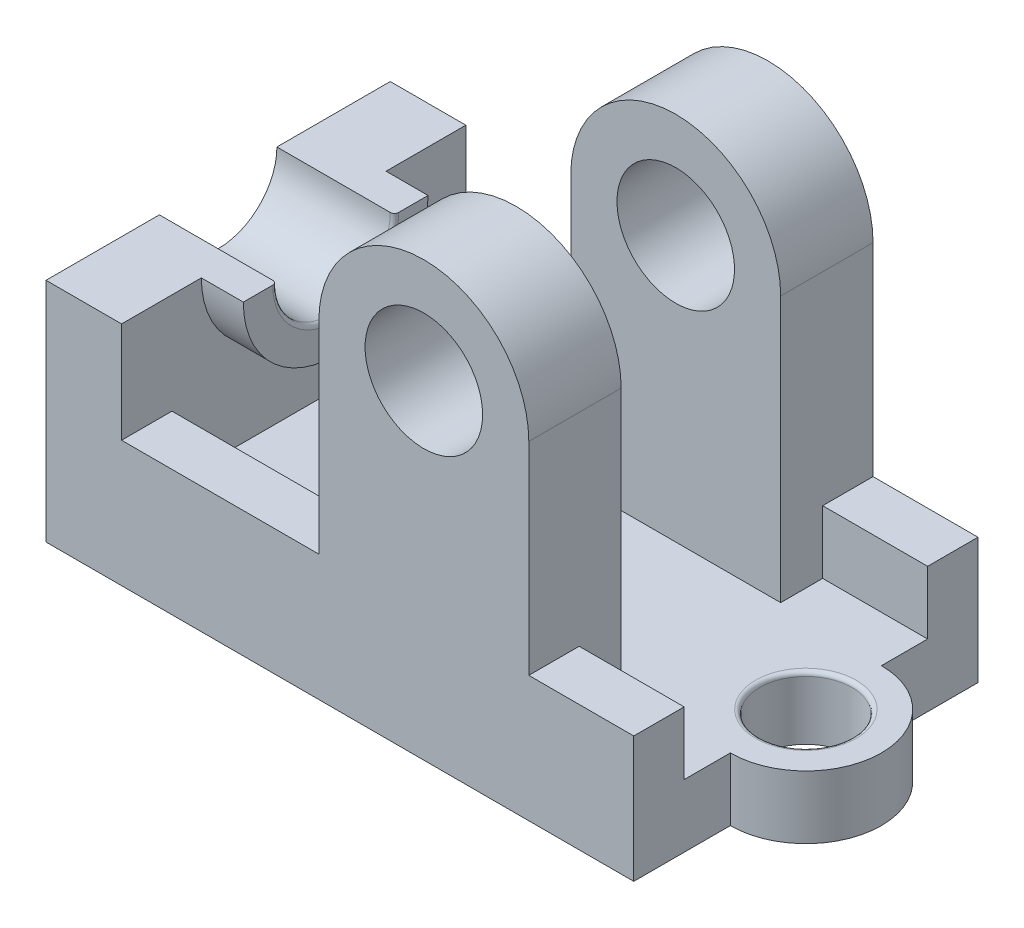
ISO-10303-21;
HEADER;
FILE_DESCRIPTION(('STEP AP214'),'2;1');
FILE_NAME('part.step','',(''),(''),'','','');
FILE_SCHEMA(('AUTOMOTIVE_DESIGN { 1 0 10303 214 1 1 1 1 }'));
ENDSEC;
DATA;
#1=APPLICATION_CONTEXT('core data for automotive mechanical design processes');
#2=APPLICATION_PROTOCOL_DEFINITION('international standard','automotive_design',2000,#1);
#3=PRODUCT_CONTEXT('',#1,'mechanical');
#4=PRODUCT('Part','Part','',(#3));
#5=PRODUCT_RELATED_PRODUCT_CATEGORY('part','',(#4));
#6=PRODUCT_DEFINITION_FORMATION('','',#4);
#7=PRODUCT_DEFINITION_CONTEXT('part definition',#1,'design');
#8=PRODUCT_DEFINITION('design','',#6,#7);
#9=PRODUCT_DEFINITION_SHAPE('','',#8);
#10=(LENGTH_UNIT() NAMED_UNIT(*) SI_UNIT(.MILLI.,.METRE.));
#11=(NAMED_UNIT(*) PLANE_ANGLE_UNIT() SI_UNIT($,.RADIAN.));
#12=(NAMED_UNIT(*) SI_UNIT($,.STERADIAN.) SOLID_ANGLE_UNIT());
#13=UNCERTAINTY_MEASURE_WITH_UNIT(LENGTH_MEASURE(1.E-05),#10,'distance_accuracy_value','');
#14=(GEOMETRIC_REPRESENTATION_CONTEXT(3) GLOBAL_UNCERTAINTY_ASSIGNED_CONTEXT((#13)) GLOBAL_UNIT_ASSIGNED_CONTEXT((#10,
#11,#12)) REPRESENTATION_CONTEXT('',''));
#15=CARTESIAN_POINT('',(0.,0.,0.));
#16=DIRECTION('',(0.,0.,1.));
#17=DIRECTION('',(1.,0.,0.));
#18=AXIS2_PLACEMENT_3D('',#15,#16,#17);
#19=CARTESIAN_POINT('',(0.,54.,0.));
#20=DIRECTION('',(0.,1.,0.));
#21=DIRECTION('',(0.,0.,1.));
#22=AXIS2_PLACEMENT_3D('',#19,#20,#21);
#23=PLANE('',#22);
#24=DIRECTION('',(-1.,0.,0.));
#25=VECTOR('',#24,1.);
#26=CARTESIAN_POINT('',(-48.,54.,-14.));
#27=LINE('',#26,#25);
#28=CARTESIAN_POINT('',(-43.,54.,-14.));
#29=VERTEX_POINT('',#28);
#30=CARTESIAN_POINT('',(-70.,54.,-14.));
#31=VERTEX_POINT('',#30);
#32=EDGE_CURVE('E460',#29,#31,#27,.T.);
#33=ORIENTED_EDGE('',*,*,#32,.F.);
#34=CARTESIAN_POINT('',(-43.,54.,-15.));
#35=DIRECTION('',(0.,1.,0.));
#36=DIRECTION('',(0.,0.,1.));
#37=AXIS2_PLACEMENT_3D('',#34,#35,#36);
#38=CIRCLE('',#37,1.);
#39=CARTESIAN_POINT('',(-42.,54.,-15.));
#40=VERTEX_POINT('',#39);
#41=EDGE_CURVE('E68',#29,#40,#38,.T.);
#42=ORIENTED_EDGE('',*,*,#41,.T.);
#43=DIRECTION('',(0.,0.,-1.));
#44=VECTOR('',#43,1.);
#45=CARTESIAN_POINT('',(-42.,54.,-14.));
#46=LINE('',#45,#44);
#47=CARTESIAN_POINT('',(-42.,54.,-22.));
#48=VERTEX_POINT('',#47);
#49=EDGE_CURVE('E234',#40,#48,#46,.T.);
#50=ORIENTED_EDGE('',*,*,#49,.T.);
#51=DIRECTION('',(-1.,0.,0.));
#52=VECTOR('',#51,1.);
#53=CARTESIAN_POINT('',(-42.,54.,-22.));
#54=LINE('',#53,#52);
#55=CARTESIAN_POINT('',(-52.,54.,-22.));
#56=VERTEX_POINT('',#55);
#57=EDGE_CURVE('E236',#48,#56,#54,.T.);
#58=ORIENTED_EDGE('',*,*,#57,.T.);
#59=DIRECTION('',(0.,0.,-1.));
#60=VECTOR('',#59,1.);
#61=CARTESIAN_POINT('',(-52.,54.,-41.));
#62=LINE('',#61,#60);
#63=CARTESIAN_POINT('',(-52.,54.,-41.));
#64=VERTEX_POINT('',#63);
#65=EDGE_CURVE('E388',#56,#64,#62,.T.);
#66=ORIENTED_EDGE('',*,*,#65,.T.);
#67=DIRECTION('',(-1.,0.,0.));
#68=VECTOR('',#67,1.);
#69=CARTESIAN_POINT('',(-70.,54.,-41.));
#70=LINE('',#69,#68);
#71=CARTESIAN_POINT('',(-70.,54.,-41.));
#72=VERTEX_POINT('',#71);
#73=EDGE_CURVE('E392',#64,#72,#70,.T.);
#74=ORIENTED_EDGE('',*,*,#73,.T.);
#75=DIRECTION('',(0.,0.,1.));
#76=VECTOR('',#75,1.);
#77=CARTESIAN_POINT('',(-70.,54.,-41.));
#78=LINE('',#77,#76);
#79=EDGE_CURVE('E381',#72,#31,#78,.T.);
#80=ORIENTED_EDGE('',*,*,#79,.T.);
#81=EDGE_LOOP('',(#33,#42,#50,#58,#66,#74,#80));
#82=FACE_BOUND('',#81,.T.);
#83=ADVANCED_FACE('F44',(#82),#23,.T.);
#84=CARTESIAN_POINT('',(-52.,30.,-29.));
#85=DIRECTION('',(0.,0.,-1.));
#86=DIRECTION('',(-1.,0.,0.));
#87=AXIS2_PLACEMENT_3D('',#84,#85,#86);
#88=PLANE('',#87);
#89=DIRECTION('',(1.,0.,0.));
#90=VECTOR('',#89,1.);
#91=CARTESIAN_POINT('',(-52.,15.,-29.));
#92=LINE('',#91,#90);
#93=CARTESIAN_POINT('',(-52.,15.,-29.));
#94=VERTEX_POINT('',#93);
#95=CARTESIAN_POINT('',(-5.,15.,-29.));
#96=VERTEX_POINT('',#95);
#97=EDGE_CURVE('E362',#94,#96,#92,.T.);
#98=ORIENTED_EDGE('',*,*,#97,.T.);
#99=DIRECTION('',(0.,1.,0.));
#100=VECTOR('',#99,1.);
#101=CARTESIAN_POINT('',(-5.,30.,-29.));
#102=LINE('',#101,#100);
#103=CARTESIAN_POINT('',(-5.,30.,-29.));
#104=VERTEX_POINT('',#103);
#105=EDGE_CURVE('E290',#96,#104,#102,.T.);
#106=ORIENTED_EDGE('',*,*,#105,.T.);
#107=DIRECTION('',(1.,0.,0.));
#108=VECTOR('',#107,1.);
#109=CARTESIAN_POINT('',(-52.,30.,-29.));
#110=LINE('',#109,#108);
#111=CARTESIAN_POINT('',(-52.,30.,-29.));
#112=VERTEX_POINT('',#111);
#113=EDGE_CURVE('E366',#112,#104,#110,.T.);
#114=ORIENTED_EDGE('',*,*,#113,.F.);
#115=DIRECTION('',(0.,-1.,0.));
#116=VECTOR('',#115,1.);
#117=CARTESIAN_POINT('',(-52.,30.,-29.));
#118=LINE('',#117,#116);
#119=EDGE_CURVE('E379',#112,#94,#118,.T.);
#120=ORIENTED_EDGE('',*,*,#119,.T.);
#121=EDGE_LOOP('',(#98,#106,#114,#120));
#122=FACE_BOUND('',#121,.T.);
#123=ADVANCED_FACE('F481',(#122),#88,.F.);
#124=CARTESIAN_POINT('',(0.,30.,0.));
#125=DIRECTION('',(0.,1.,0.));
#126=DIRECTION('',(0.,0.,1.));
#127=AXIS2_PLACEMENT_3D('',#124,#125,#126);
#128=PLANE('',#127);
#129=DIRECTION('',(0.,0.,1.));
#130=VECTOR('',#129,1.);
#131=CARTESIAN_POINT('',(-5.,30.,0.));
#132=LINE('',#131,#130);
#133=CARTESIAN_POINT('',(-5.,30.,-41.));
#134=VERTEX_POINT('',#133);
#135=EDGE_CURVE('E452',#134,#104,#132,.T.);
#136=ORIENTED_EDGE('',*,*,#135,.F.);
#137=DIRECTION('',(-1.,0.,0.));
#138=VECTOR('',#137,1.);
#139=CARTESIAN_POINT('',(-52.,30.,-41.));
#140=LINE('',#139,#138);
#141=CARTESIAN_POINT('',(-52.,30.,-41.));
#142=VERTEX_POINT('',#141);
#143=EDGE_CURVE('E375',#134,#142,#140,.T.);
#144=ORIENTED_EDGE('',*,*,#143,.T.);
#145=DIRECTION('',(0.,0.,1.));
#146=VECTOR('',#145,1.);
#147=CARTESIAN_POINT('',(-52.,30.,-41.));
#148=LINE('',#147,#146);
#149=EDGE_CURVE('E363',#142,#112,#148,.T.);
#150=ORIENTED_EDGE('',*,*,#149,.T.);
#151=ORIENTED_EDGE('',*,*,#113,.T.);
#152=EDGE_LOOP('',(#136,#144,#150,#151));
#153=FACE_BOUND('',#152,.T.);
#154=ADVANCED_FACE('F490',(#153),#128,.T.);
#155=CARTESIAN_POINT('',(-52.,30.,29.));
#156=DIRECTION('',(0.,0.,1.));
#157=DIRECTION('',(1.,0.,0.));
#158=AXIS2_PLACEMENT_3D('',#155,#156,#157);
#159=PLANE('',#158);
#160=DIRECTION('',(-1.,0.,0.));
#161=VECTOR('',#160,1.);
#162=CARTESIAN_POINT('',(-52.,15.,29.));
#163=LINE('',#162,#161);
#164=CARTESIAN_POINT('',(70.,15.,29.));
#165=VERTEX_POINT('',#164);
#166=CARTESIAN_POINT('',(45.,15.,29.));
#167=VERTEX_POINT('',#166);
#168=EDGE_CURVE('E344',#165,#167,#163,.T.);
#169=ORIENTED_EDGE('',*,*,#168,.T.);
#170=DIRECTION('',(0.,1.,0.));
#171=VECTOR('',#170,1.);
#172=CARTESIAN_POINT('',(45.,30.,29.));
#173=LINE('',#172,#171);
#174=CARTESIAN_POINT('',(45.,30.,29.));
#175=VERTEX_POINT('',#174);
#176=EDGE_CURVE('E331',#167,#175,#173,.T.);
#177=ORIENTED_EDGE('',*,*,#176,.T.);
#178=DIRECTION('',(-1.,0.,0.));
#179=VECTOR('',#178,1.);
#180=CARTESIAN_POINT('',(-52.,30.,29.));
#181=LINE('',#180,#179);
#182=CARTESIAN_POINT('',(70.,30.,29.));
#183=VERTEX_POINT('',#182);
#184=EDGE_CURVE('E347',#183,#175,#181,.T.);
#185=ORIENTED_EDGE('',*,*,#184,.F.);
#186=DIRECTION('',(0.,-1.,0.));
#187=VECTOR('',#186,1.);
#188=CARTESIAN_POINT('',(70.,30.,29.));
#189=LINE('',#188,#187);
#190=EDGE_CURVE('E357',#183,#165,#189,.T.);
#191=ORIENTED_EDGE('',*,*,#190,.T.);
#192=EDGE_LOOP('',(#169,#177,#185,#191));
#193=FACE_BOUND('',#192,.T.);
#194=ADVANCED_FACE('F575',(#193),#159,.F.);
#195=CARTESIAN_POINT('',(0.,30.,0.));
#196=DIRECTION('',(0.,-1.,0.));
#197=DIRECTION('',(0.,0.,-1.));
#198=AXIS2_PLACEMENT_3D('',#195,#196,#197);
#199=PLANE('',#198);
#200=ORIENTED_EDGE('',*,*,#184,.T.);
#201=DIRECTION('',(0.,0.,1.));
#202=VECTOR('',#201,1.);
#203=CARTESIAN_POINT('',(45.,30.,0.));
#204=LINE('',#203,#202);
#205=CARTESIAN_POINT('',(45.,30.,41.));
#206=VERTEX_POINT('',#205);
#207=EDGE_CURVE('E444',#175,#206,#204,.T.);
#208=ORIENTED_EDGE('',*,*,#207,.T.);
#209=DIRECTION('',(1.,0.,0.));
#210=VECTOR('',#209,1.);
#211=CARTESIAN_POINT('',(-52.,30.,41.));
#212=LINE('',#211,#210);
#213=CARTESIAN_POINT('',(70.,30.,41.));
#214=VERTEX_POINT('',#213);
#215=EDGE_CURVE('E345',#206,#214,#212,.T.);
#216=ORIENTED_EDGE('',*,*,#215,.T.);
#217=DIRECTION('',(0.,0.,-1.));
#218=VECTOR('',#217,1.);
#219=CARTESIAN_POINT('',(70.,30.,41.));
#220=LINE('',#219,#218);
#221=EDGE_CURVE('E346',#214,#183,#220,.T.);
#222=ORIENTED_EDGE('',*,*,#221,.T.);
#223=EDGE_LOOP('',(#200,#208,#216,#222));
#224=FACE_BOUND('',#223,.T.);
#225=ADVANCED_FACE('F547',(#224),#199,.F.);
#226=CARTESIAN_POINT('',(70.,15.,0.));
#227=DIRECTION('',(0.,1.,0.));
#228=DIRECTION('',(0.,0.,1.));
#229=AXIS2_PLACEMENT_3D('',#226,#227,#228);
#230=PLANE('',#229);
#231=CARTESIAN_POINT('',(70.,15.,0.));
#232=DIRECTION('',(0.,1.,0.));
#233=DIRECTION('',(0.,0.,1.));
#234=AXIS2_PLACEMENT_3D('',#231,#232,#233);
#235=CIRCLE('',#234,12.);
#236=CARTESIAN_POINT('',(70.,15.,12.));
#237=VERTEX_POINT('',#236);
#238=EDGE_CURVE('E11',#237,#237,#235,.F.);
#239=ORIENTED_EDGE('',*,*,#238,.T.);
#240=EDGE_LOOP('',(#239));
#241=FACE_BOUND('',#240,.T.);
#242=DIRECTION('',(0.,0.,1.));
#243=VECTOR('',#242,1.);
#244=CARTESIAN_POINT('',(-5.,15.,0.));
#245=LINE('',#244,#243);
#246=CARTESIAN_POINT('',(-5.,15.,-19.));
#247=VERTEX_POINT('',#246);
#248=EDGE_CURVE('E292',#96,#247,#245,.T.);
#249=ORIENTED_EDGE('',*,*,#248,.F.);
#250=ORIENTED_EDGE('',*,*,#97,.F.);
#251=DIRECTION('',(0.,0.,-1.));
#252=VECTOR('',#251,1.);
#253=CARTESIAN_POINT('',(-52.,15.,-41.));
#254=LINE('',#253,#252);
#255=CARTESIAN_POINT('',(-52.,15.,29.));
#256=VERTEX_POINT('',#255);
#257=EDGE_CURVE('E384',#256,#94,#254,.T.);
#258=ORIENTED_EDGE('',*,*,#257,.F.);
#259=CARTESIAN_POINT('',(-5.,15.,29.));
#260=VERTEX_POINT('',#259);
#261=EDGE_CURVE('E336',#260,#256,#163,.T.);
#262=ORIENTED_EDGE('',*,*,#261,.F.);
#263=DIRECTION('',(0.,0.,1.));
#264=VECTOR('',#263,1.);
#265=CARTESIAN_POINT('',(-5.,15.,0.));
#266=LINE('',#265,#264);
#267=CARTESIAN_POINT('',(-5.,15.,19.));
#268=VERTEX_POINT('',#267);
#269=EDGE_CURVE('E328',#268,#260,#266,.T.);
#270=ORIENTED_EDGE('',*,*,#269,.F.);
#271=DIRECTION('',(1.,0.,0.));
#272=VECTOR('',#271,1.);
#273=CARTESIAN_POINT('',(70.,15.,19.));
#274=LINE('',#273,#272);
#275=CARTESIAN_POINT('',(45.,15.,19.));
#276=VERTEX_POINT('',#275);
#277=EDGE_CURVE('E337',#268,#276,#274,.T.);
#278=ORIENTED_EDGE('',*,*,#277,.T.);
#279=DIRECTION('',(0.,0.,-1.));
#280=VECTOR('',#279,1.);
#281=CARTESIAN_POINT('',(45.,15.,0.));
#282=LINE('',#281,#280);
#283=EDGE_CURVE('E334',#167,#276,#282,.T.);
#284=ORIENTED_EDGE('',*,*,#283,.F.);
#285=ORIENTED_EDGE('',*,*,#168,.F.);
#286=DIRECTION('',(0.,0.,-1.));
#287=VECTOR('',#286,1.);
#288=CARTESIAN_POINT('',(70.,15.,18.));
#289=LINE('',#288,#287);
#290=CARTESIAN_POINT('',(70.,15.,18.));
#291=VERTEX_POINT('',#290);
#292=EDGE_CURVE('E410',#165,#291,#289,.T.);
#293=ORIENTED_EDGE('',*,*,#292,.T.);
#294=CARTESIAN_POINT('',(70.,15.,0.));
#295=DIRECTION('',(0.,1.,0.));
#296=DIRECTION('',(0.,0.,1.));
#297=AXIS2_PLACEMENT_3D('',#294,#295,#296);
#298=CIRCLE('',#297,18.);
#299=CARTESIAN_POINT('',(70.,15.,-18.));
#300=VERTEX_POINT('',#299);
#301=EDGE_CURVE('E406',#291,#300,#298,.T.);
#302=ORIENTED_EDGE('',*,*,#301,.T.);
#303=DIRECTION('',(0.,0.,-1.));
#304=VECTOR('',#303,1.);
#305=CARTESIAN_POINT('',(70.,15.,-41.));
#306=LINE('',#305,#304);
#307=CARTESIAN_POINT('',(70.,15.,-29.));
#308=VERTEX_POINT('',#307);
#309=EDGE_CURVE('E415',#300,#308,#306,.T.);
#310=ORIENTED_EDGE('',*,*,#309,.T.);
#311=CARTESIAN_POINT('',(45.,15.,-29.));
#312=VERTEX_POINT('',#311);
#313=EDGE_CURVE('E359',#312,#308,#92,.T.);
#314=ORIENTED_EDGE('',*,*,#313,.F.);
#315=DIRECTION('',(0.,0.,-1.));
#316=VECTOR('',#315,1.);
#317=CARTESIAN_POINT('',(45.,15.,0.));
#318=LINE('',#317,#316);
#319=CARTESIAN_POINT('',(45.,15.,-19.));
#320=VERTEX_POINT('',#319);
#321=EDGE_CURVE('E287',#320,#312,#318,.T.);
#322=ORIENTED_EDGE('',*,*,#321,.F.);
#323=DIRECTION('',(1.,0.,0.));
#324=VECTOR('',#323,1.);
#325=CARTESIAN_POINT('',(70.,15.,-19.));
#326=LINE('',#325,#324);
#327=EDGE_CURVE('E294',#247,#320,#326,.T.);
#328=ORIENTED_EDGE('',*,*,#327,.F.);
#329=EDGE_LOOP('',(#249,#250,#258,#262,#270,#278,#284,#285,#293,#302,#310,#314,#322,#328));
#330=FACE_BOUND('',#329,.T.);
#331=ADVANCED_FACE('F568',(#241,#330),#230,.T.);
#332=CARTESIAN_POINT('',(-52.,54.,-41.));
#333=DIRECTION('',(-1.,0.,0.));
#334=DIRECTION('',(0.,0.,1.));
#335=AXIS2_PLACEMENT_3D('',#332,#333,#334);
#336=PLANE('',#335);
#337=ORIENTED_EDGE('',*,*,#65,.F.);
#338=CARTESIAN_POINT('',(-52.,54.,0.));
#339=DIRECTION('',(-1.,0.,0.));
#340=DIRECTION('',(0.,0.,1.));
#341=AXIS2_PLACEMENT_3D('',#338,#339,#340);
#342=CIRCLE('',#341,22.);
#343=CARTESIAN_POINT('',(-52.,54.,22.));
#344=VERTEX_POINT('',#343);
#345=EDGE_CURVE('E244',#56,#344,#342,.T.);
#346=ORIENTED_EDGE('',*,*,#345,.T.);
#347=CARTESIAN_POINT('',(-52.,54.,41.));
#348=VERTEX_POINT('',#347);
#349=EDGE_CURVE('E391',#348,#344,#62,.T.);
#350=ORIENTED_EDGE('',*,*,#349,.F.);
#351=DIRECTION('',(0.,-1.,0.));
#352=VECTOR('',#351,1.);
#353=CARTESIAN_POINT('',(-52.,54.,41.));
#354=LINE('',#353,#352);
#355=CARTESIAN_POINT('',(-52.,30.,41.));
#356=VERTEX_POINT('',#355);
#357=EDGE_CURVE('E402',#348,#356,#354,.T.);
#358=ORIENTED_EDGE('',*,*,#357,.T.);
#359=DIRECTION('',(0.,0.,1.));
#360=VECTOR('',#359,1.);
#361=CARTESIAN_POINT('',(-52.,30.,41.));
#362=LINE('',#361,#360);
#363=CARTESIAN_POINT('',(-52.,30.,29.));
#364=VERTEX_POINT('',#363);
#365=EDGE_CURVE('E339',#364,#356,#362,.T.);
#366=ORIENTED_EDGE('',*,*,#365,.F.);
#367=DIRECTION('',(0.,-1.,0.));
#368=VECTOR('',#367,1.);
#369=CARTESIAN_POINT('',(-52.,30.,29.));
#370=LINE('',#369,#368);
#371=EDGE_CURVE('E352',#364,#256,#370,.T.);
#372=ORIENTED_EDGE('',*,*,#371,.T.);
#373=ORIENTED_EDGE('',*,*,#257,.T.);
#374=ORIENTED_EDGE('',*,*,#119,.F.);
#375=ORIENTED_EDGE('',*,*,#149,.F.);
#376=DIRECTION('',(0.,-1.,0.));
#377=VECTOR('',#376,1.);
#378=CARTESIAN_POINT('',(-52.,54.,-41.));
#379=LINE('',#378,#377);
#380=EDGE_CURVE('E397',#64,#142,#379,.T.);
#381=ORIENTED_EDGE('',*,*,#380,.F.);
#382=EDGE_LOOP('',(#337,#346,#350,#358,#366,#372,#373,#374,#375,#381));
#383=FACE_BOUND('',#382,.T.);
#384=ADVANCED_FACE('F526',(#383),#336,.F.);
#385=CARTESIAN_POINT('',(70.,0.,0.));
#386=DIRECTION('',(0.,1.,0.));
#387=DIRECTION('',(0.,0.,1.));
#388=AXIS2_PLACEMENT_3D('',#385,#386,#387);
#389=PLANE('',#388);
#390=DIRECTION('',(0.,0.,1.));
#391=VECTOR('',#390,1.);
#392=CARTESIAN_POINT('',(-70.,0.,-41.));
#393=LINE('',#392,#391);
#394=CARTESIAN_POINT('',(-70.,0.,-41.));
#395=VERTEX_POINT('',#394);
#396=CARTESIAN_POINT('',(-70.,0.,41.));
#397=VERTEX_POINT('',#396);
#398=EDGE_CURVE('E408',#395,#397,#393,.T.);
#399=ORIENTED_EDGE('',*,*,#398,.F.);
#400=DIRECTION('',(-1.,0.,0.));
#401=VECTOR('',#400,1.);
#402=CARTESIAN_POINT('',(-70.,0.,-41.));
#403=LINE('',#402,#401);
#404=CARTESIAN_POINT('',(70.,0.,-41.));
#405=VERTEX_POINT('',#404);
#406=EDGE_CURVE('E421',#405,#395,#403,.T.);
#407=ORIENTED_EDGE('',*,*,#406,.F.);
#408=DIRECTION('',(0.,0.,-1.));
#409=VECTOR('',#408,1.);
#410=CARTESIAN_POINT('',(70.,0.,-41.));
#411=LINE('',#410,#409);
#412=CARTESIAN_POINT('',(70.,0.,-18.));
#413=VERTEX_POINT('',#412);
#414=EDGE_CURVE('E423',#413,#405,#411,.T.);
#415=ORIENTED_EDGE('',*,*,#414,.F.);
#416=CARTESIAN_POINT('',(70.,0.,0.));
#417=DIRECTION('',(0.,1.,0.));
#418=DIRECTION('',(0.,0.,1.));
#419=AXIS2_PLACEMENT_3D('',#416,#417,#418);
#420=CIRCLE('',#419,18.);
#421=CARTESIAN_POINT('',(70.,0.,18.));
#422=VERTEX_POINT('',#421);
#423=EDGE_CURVE('E418',#422,#413,#420,.T.);
#424=ORIENTED_EDGE('',*,*,#423,.F.);
#425=DIRECTION('',(0.,0.,-1.));
#426=VECTOR('',#425,1.);
#427=CARTESIAN_POINT('',(70.,0.,18.));
#428=LINE('',#427,#426);
#429=CARTESIAN_POINT('',(70.,0.,41.));
#430=VERTEX_POINT('',#429);
#431=EDGE_CURVE('E417',#430,#422,#428,.T.);
#432=ORIENTED_EDGE('',*,*,#431,.F.);
#433=DIRECTION('',(1.,0.,0.));
#434=VECTOR('',#433,1.);
#435=CARTESIAN_POINT('',(-70.,0.,41.));
#436=LINE('',#435,#434);
#437=EDGE_CURVE('E407',#397,#430,#436,.T.);
#438=ORIENTED_EDGE('',*,*,#437,.F.);
#439=EDGE_LOOP('',(#399,#407,#415,#424,#432,#438));
#440=FACE_BOUND('',#439,.T.);
#441=CARTESIAN_POINT('',(70.,0.,0.));
#442=DIRECTION('',(0.,1.,0.));
#443=DIRECTION('',(0.,0.,1.));
#444=AXIS2_PLACEMENT_3D('',#441,#442,#443);
#445=CIRCLE('',#444,11.);
#446=CARTESIAN_POINT('',(70.,0.,11.));
#447=VERTEX_POINT('',#446);
#448=EDGE_CURVE('E401',#447,#447,#445,.T.);
#449=ORIENTED_EDGE('',*,*,#448,.T.);
#450=EDGE_LOOP('',(#449));
#451=FACE_BOUND('',#450,.T.);
#452=ADVANCED_FACE('F533',(#440,#451),#389,.F.);
#453=CARTESIAN_POINT('',(-70.,15.,41.));
#454=DIRECTION('',(0.,0.,-1.));
#455=DIRECTION('',(-1.,0.,0.));
#456=AXIS2_PLACEMENT_3D('',#453,#454,#455);
#457=PLANE('',#456);
#458=ORIENTED_EDGE('',*,*,#437,.T.);
#459=DIRECTION('',(0.,-1.,0.));
#460=VECTOR('',#459,1.);
#461=CARTESIAN_POINT('',(70.,15.,41.));
#462=LINE('',#461,#460);
#463=EDGE_CURVE('E439',#214,#430,#462,.T.);
#464=ORIENTED_EDGE('',*,*,#463,.F.);
#465=ORIENTED_EDGE('',*,*,#215,.F.);
#466=DIRECTION('',(0.,1.,0.));
#467=VECTOR('',#466,1.);
#468=CARTESIAN_POINT('',(45.,78.2547922733362,41.));
#469=LINE('',#468,#467);
#470=CARTESIAN_POINT('',(45.,78.2547922733362,41.));
#471=VERTEX_POINT('',#470);
#472=EDGE_CURVE('E307',#206,#471,#469,.T.);
#473=ORIENTED_EDGE('',*,*,#472,.T.);
#474=CARTESIAN_POINT('',(20.,78.2547922733362,41.));
#475=DIRECTION('',(0.,0.,1.));
#476=DIRECTION('',(1.,0.,0.));
#477=AXIS2_PLACEMENT_3D('',#474,#475,#476);
#478=CIRCLE('',#477,25.);
#479=CARTESIAN_POINT('',(-5.,78.2547922733362,41.));
#480=VERTEX_POINT('',#479);
#481=EDGE_CURVE('E305',#471,#480,#478,.T.);
#482=ORIENTED_EDGE('',*,*,#481,.T.);
#483=DIRECTION('',(0.,-1.,0.));
#484=VECTOR('',#483,1.);
#485=CARTESIAN_POINT('',(-5.,30.,41.));
#486=LINE('',#485,#484);
#487=CARTESIAN_POINT('',(-5.,30.,41.));
#488=VERTEX_POINT('',#487);
#489=EDGE_CURVE('E320',#480,#488,#486,.T.);
#490=ORIENTED_EDGE('',*,*,#489,.T.);
#491=EDGE_CURVE('E341',#356,#488,#212,.T.);
#492=ORIENTED_EDGE('',*,*,#491,.F.);
#493=ORIENTED_EDGE('',*,*,#357,.F.);
#494=DIRECTION('',(1.,0.,0.));
#495=VECTOR('',#494,1.);
#496=CARTESIAN_POINT('',(-70.,54.,41.));
#497=LINE('',#496,#495);
#498=CARTESIAN_POINT('',(-70.,54.,41.));
#499=VERTEX_POINT('',#498);
#500=EDGE_CURVE('E390',#499,#348,#497,.T.);
#501=ORIENTED_EDGE('',*,*,#500,.F.);
#502=DIRECTION('',(0.,-1.,0.));
#503=VECTOR('',#502,1.);
#504=CARTESIAN_POINT('',(-70.,15.,41.));
#505=LINE('',#504,#503);
#506=EDGE_CURVE('E414',#499,#397,#505,.T.);
#507=ORIENTED_EDGE('',*,*,#506,.T.);
#508=EDGE_LOOP('',(#458,#464,#465,#473,#482,#490,#492,#493,#501,#507));
#509=FACE_BOUND('',#508,.T.);
#510=CARTESIAN_POINT('',(20.,78.2547922733362,41.));
#511=DIRECTION('',(0.,0.,1.));
#512=DIRECTION('',(1.,0.,0.));
#513=AXIS2_PLACEMENT_3D('',#510,#511,#512);
#514=CIRCLE('',#513,14.);
#515=CARTESIAN_POINT('',(34.,78.2547922733362,41.));
#516=VERTEX_POINT('',#515);
#517=EDGE_CURVE('E296',#516,#516,#514,.T.);
#518=ORIENTED_EDGE('',*,*,#517,.F.);
#519=EDGE_LOOP('',(#518));
#520=FACE_BOUND('',#519,.T.);
#521=ADVANCED_FACE('F518',(#509,#520),#457,.F.);
#522=CARTESIAN_POINT('',(70.,15.,18.));
#523=DIRECTION('',(-1.,0.,0.));
#524=DIRECTION('',(0.,0.,1.));
#525=AXIS2_PLACEMENT_3D('',#522,#523,#524);
#526=PLANE('',#525);
#527=ORIENTED_EDGE('',*,*,#431,.T.);
#528=DIRECTION('',(0.,-1.,0.));
#529=VECTOR('',#528,1.);
#530=CARTESIAN_POINT('',(70.,15.,18.));
#531=LINE('',#530,#529);
#532=EDGE_CURVE('E440',#291,#422,#531,.T.);
#533=ORIENTED_EDGE('',*,*,#532,.F.);
#534=ORIENTED_EDGE('',*,*,#292,.F.);
#535=ORIENTED_EDGE('',*,*,#190,.F.);
#536=ORIENTED_EDGE('',*,*,#221,.F.);
#537=ORIENTED_EDGE('',*,*,#463,.T.);
#538=EDGE_LOOP('',(#527,#533,#534,#535,#536,#537));
#539=FACE_BOUND('',#538,.T.);
#540=ADVANCED_FACE('F542',(#539),#526,.F.);
#541=CARTESIAN_POINT('',(70.,15.,0.));
#542=DIRECTION('',(0.,-1.,0.));
#543=DIRECTION('',(0.,0.,-1.));
#544=AXIS2_PLACEMENT_3D('',#541,#542,#543);
#545=CYLINDRICAL_SURFACE('',#544,18.);
#546=ORIENTED_EDGE('',*,*,#423,.T.);
#547=DIRECTION('',(0.,-1.,0.));
#548=VECTOR('',#547,1.);
#549=CARTESIAN_POINT('',(70.,15.,-18.));
#550=LINE('',#549,#548);
#551=EDGE_CURVE('E432',#300,#413,#550,.T.);
#552=ORIENTED_EDGE('',*,*,#551,.F.);
#553=ORIENTED_EDGE('',*,*,#301,.F.);
#554=ORIENTED_EDGE('',*,*,#532,.T.);
#555=EDGE_LOOP('',(#546,#552,#553,#554));
#556=FACE_BOUND('',#555,.T.);
#557=ADVANCED_FACE('F580',(#556),#545,.T.);
#558=CARTESIAN_POINT('',(70.,15.,-41.));
#559=DIRECTION('',(-1.,0.,0.));
#560=DIRECTION('',(0.,0.,1.));
#561=AXIS2_PLACEMENT_3D('',#558,#559,#560);
#562=PLANE('',#561);
#563=ORIENTED_EDGE('',*,*,#414,.T.);
#564=DIRECTION('',(0.,-1.,0.));
#565=VECTOR('',#564,1.);
#566=CARTESIAN_POINT('',(70.,15.,-41.));
#567=LINE('',#566,#565);
#568=CARTESIAN_POINT('',(70.,30.,-41.));
#569=VERTEX_POINT('',#568);
#570=EDGE_CURVE('E431',#569,#405,#567,.T.);
#571=ORIENTED_EDGE('',*,*,#570,.F.);
#572=DIRECTION('',(0.,0.,-1.));
#573=VECTOR('',#572,1.);
#574=CARTESIAN_POINT('',(70.,30.,-41.));
#575=LINE('',#574,#573);
#576=CARTESIAN_POINT('',(70.,30.,-29.));
#577=VERTEX_POINT('',#576);
#578=EDGE_CURVE('E367',#577,#569,#575,.T.);
#579=ORIENTED_EDGE('',*,*,#578,.F.);
#580=DIRECTION('',(0.,-1.,0.));
#581=VECTOR('',#580,1.);
#582=CARTESIAN_POINT('',(70.,30.,-29.));
#583=LINE('',#582,#581);
#584=EDGE_CURVE('E374',#577,#308,#583,.T.);
#585=ORIENTED_EDGE('',*,*,#584,.T.);
#586=ORIENTED_EDGE('',*,*,#309,.F.);
#587=ORIENTED_EDGE('',*,*,#551,.T.);
#588=EDGE_LOOP('',(#563,#571,#579,#585,#586,#587));
#589=FACE_BOUND('',#588,.T.);
#590=ADVANCED_FACE('F578',(#589),#562,.F.);
#591=CARTESIAN_POINT('',(-70.,15.,-41.));
#592=DIRECTION('',(0.,0.,1.));
#593=DIRECTION('',(1.,0.,0.));
#594=AXIS2_PLACEMENT_3D('',#591,#592,#593);
#595=PLANE('',#594);
#596=ORIENTED_EDGE('',*,*,#406,.T.);
#597=DIRECTION('',(0.,-1.,0.));
#598=VECTOR('',#597,1.);
#599=CARTESIAN_POINT('',(-70.,15.,-41.));
#600=LINE('',#599,#598);
#601=EDGE_CURVE('E426',#72,#395,#600,.T.);
#602=ORIENTED_EDGE('',*,*,#601,.F.);
#603=ORIENTED_EDGE('',*,*,#73,.F.);
#604=ORIENTED_EDGE('',*,*,#380,.T.);
#605=ORIENTED_EDGE('',*,*,#143,.F.);
#606=DIRECTION('',(0.,1.,0.));
#607=VECTOR('',#606,1.);
#608=CARTESIAN_POINT('',(-5.,0.,-41.));
#609=LINE('',#608,#607);
#610=CARTESIAN_POINT('',(-5.,78.2547922733362,-41.));
#611=VERTEX_POINT('',#610);
#612=EDGE_CURVE('E268',#134,#611,#609,.T.);
#613=ORIENTED_EDGE('',*,*,#612,.T.);
#614=CARTESIAN_POINT('',(20.,78.2547922733362,-41.));
#615=DIRECTION('',(0.,0.,-1.));
#616=DIRECTION('',(1.,0.,0.));
#617=AXIS2_PLACEMENT_3D('',#614,#615,#616);
#618=CIRCLE('',#617,25.);
#619=CARTESIAN_POINT('',(45.,78.254792273336,-41.));
#620=VERTEX_POINT('',#619);
#621=EDGE_CURVE('E265',#611,#620,#618,.T.);
#622=ORIENTED_EDGE('',*,*,#621,.T.);
#623=DIRECTION('',(0.,-1.,0.));
#624=VECTOR('',#623,1.);
#625=CARTESIAN_POINT('',(45.,78.254792273336,-41.));
#626=LINE('',#625,#624);
#627=CARTESIAN_POINT('',(45.,30.,-41.));
#628=VERTEX_POINT('',#627);
#629=EDGE_CURVE('E280',#620,#628,#626,.T.);
#630=ORIENTED_EDGE('',*,*,#629,.T.);
#631=EDGE_CURVE('E373',#569,#628,#140,.T.);
#632=ORIENTED_EDGE('',*,*,#631,.F.);
#633=ORIENTED_EDGE('',*,*,#570,.T.);
#634=EDGE_LOOP('',(#596,#602,#603,#604,#605,#613,#622,#630,#632,#633));
#635=FACE_BOUND('',#634,.T.);
#636=CARTESIAN_POINT('',(20.,78.2547922733362,-41.));
#637=DIRECTION('',(0.,0.,-1.));
#638=DIRECTION('',(-1.,0.,0.));
#639=AXIS2_PLACEMENT_3D('',#636,#637,#638);
#640=CIRCLE('',#639,14.);
#641=CARTESIAN_POINT('',(6.00000000000001,78.2547922733362,-41.));
#642=VERTEX_POINT('',#641);
#643=EDGE_CURVE('E259',#642,#642,#640,.T.);
#644=ORIENTED_EDGE('',*,*,#643,.F.);
#645=EDGE_LOOP('',(#644));
#646=FACE_BOUND('',#645,.T.);
#647=ADVANCED_FACE('F532',(#635,#646),#595,.F.);
#648=CARTESIAN_POINT('',(-70.,15.,-41.));
#649=DIRECTION('',(1.,0.,0.));
#650=DIRECTION('',(0.,0.,-1.));
#651=AXIS2_PLACEMENT_3D('',#648,#649,#650);
#652=PLANE('',#651);
#653=ORIENTED_EDGE('',*,*,#506,.F.);
#654=CARTESIAN_POINT('',(-70.,54.,14.));
#655=VERTEX_POINT('',#654);
#656=EDGE_CURVE('E389',#655,#499,#78,.T.);
#657=ORIENTED_EDGE('',*,*,#656,.F.);
#658=CARTESIAN_POINT('',(-70.,54.,0.));
#659=DIRECTION('',(-1.,0.,0.));
#660=DIRECTION('',(0.,0.,1.));
#661=AXIS2_PLACEMENT_3D('',#658,#659,#660);
#662=CIRCLE('',#661,14.);
#663=EDGE_CURVE('E257',#31,#655,#662,.T.);
#664=ORIENTED_EDGE('',*,*,#663,.F.);
#665=ORIENTED_EDGE('',*,*,#79,.F.);
#666=ORIENTED_EDGE('',*,*,#601,.T.);
#667=ORIENTED_EDGE('',*,*,#398,.T.);
#668=EDGE_LOOP('',(#653,#657,#664,#665,#666,#667));
#669=FACE_BOUND('',#668,.T.);
#670=ADVANCED_FACE('F505',(#669),#652,.F.);
#671=CARTESIAN_POINT('',(70.,15.,0.));
#672=DIRECTION('',(0.,-1.,0.));
#673=DIRECTION('',(0.,0.,-1.));
#674=AXIS2_PLACEMENT_3D('',#671,#672,#673);
#675=CYLINDRICAL_SURFACE('',#674,11.);
#676=CARTESIAN_POINT('',(70.,14.,0.));
#677=DIRECTION('',(0.,1.,0.));
#678=DIRECTION('',(0.,0.,1.));
#679=AXIS2_PLACEMENT_3D('',#676,#677,#678);
#680=CIRCLE('',#679,11.);
#681=CARTESIAN_POINT('',(70.,14.,11.));
#682=VERTEX_POINT('',#681);
#683=EDGE_CURVE('E52',#682,#682,#680,.T.);
#684=ORIENTED_EDGE('',*,*,#683,.T.);
#685=EDGE_LOOP('',(#684));
#686=FACE_BOUND('',#685,.T.);
#687=ORIENTED_EDGE('',*,*,#448,.F.);
#688=EDGE_LOOP('',(#687));
#689=FACE_BOUND('',#688,.T.);
#690=ADVANCED_FACE('F466',(#686,#689),#675,.F.);
#691=DIRECTION('',(0.,0.,-1.));
#692=VECTOR('',#691,1.);
#693=CARTESIAN_POINT('',(-42.,54.,14.));
#694=LINE('',#693,#692);
#695=CARTESIAN_POINT('',(-42.,54.,22.));
#696=VERTEX_POINT('',#695);
#697=CARTESIAN_POINT('',(-42.,54.,15.));
#698=VERTEX_POINT('',#697);
#699=EDGE_CURVE('E247',#696,#698,#694,.T.);
#700=ORIENTED_EDGE('',*,*,#699,.T.);
#701=CARTESIAN_POINT('',(-43.,54.,15.));
#702=DIRECTION('',(0.,1.,0.));
#703=DIRECTION('',(0.,0.,1.));
#704=AXIS2_PLACEMENT_3D('',#701,#702,#703);
#705=CIRCLE('',#704,1.);
#706=CARTESIAN_POINT('',(-43.,54.,14.));
#707=VERTEX_POINT('',#706);
#708=EDGE_CURVE('E463',#698,#707,#705,.T.);
#709=ORIENTED_EDGE('',*,*,#708,.T.);
#710=DIRECTION('',(-1.,0.,0.));
#711=VECTOR('',#710,1.);
#712=CARTESIAN_POINT('',(-48.,54.,14.));
#713=LINE('',#712,#711);
#714=EDGE_CURVE('E451',#655,#707,#713,.F.);
#715=ORIENTED_EDGE('',*,*,#714,.F.);
#716=ORIENTED_EDGE('',*,*,#656,.T.);
#717=ORIENTED_EDGE('',*,*,#500,.T.);
#718=ORIENTED_EDGE('',*,*,#349,.T.);
#719=DIRECTION('',(-1.,0.,0.));
#720=VECTOR('',#719,1.);
#721=CARTESIAN_POINT('',(-42.,54.,22.));
#722=LINE('',#721,#720);
#723=EDGE_CURVE('E250',#696,#344,#722,.T.);
#724=ORIENTED_EDGE('',*,*,#723,.F.);
#725=EDGE_LOOP('',(#700,#709,#715,#716,#717,#718,#724));
#726=FACE_BOUND('',#725,.T.);
#727=ADVANCED_FACE('F484',(#726),#23,.T.);
#728=CARTESIAN_POINT('',(45.,30.,-29.));
#729=VERTEX_POINT('',#728);
#730=EDGE_CURVE('E364',#729,#577,#110,.T.);
#731=ORIENTED_EDGE('',*,*,#730,.F.);
#732=DIRECTION('',(0.,-1.,0.));
#733=VECTOR('',#732,1.);
#734=CARTESIAN_POINT('',(45.,30.,-29.));
#735=LINE('',#734,#733);
#736=EDGE_CURVE('E282',#729,#312,#735,.T.);
#737=ORIENTED_EDGE('',*,*,#736,.T.);
#738=ORIENTED_EDGE('',*,*,#313,.T.);
#739=ORIENTED_EDGE('',*,*,#584,.F.);
#740=EDGE_LOOP('',(#731,#737,#738,#739));
#741=FACE_BOUND('',#740,.T.);
#742=ADVANCED_FACE('F495',(#741),#88,.F.);
#743=DIRECTION('',(0.,0.,-1.));
#744=VECTOR('',#743,1.);
#745=CARTESIAN_POINT('',(45.,30.,0.));
#746=LINE('',#745,#744);
#747=EDGE_CURVE('E449',#729,#628,#746,.T.);
#748=ORIENTED_EDGE('',*,*,#747,.F.);
#749=ORIENTED_EDGE('',*,*,#730,.T.);
#750=ORIENTED_EDGE('',*,*,#578,.T.);
#751=ORIENTED_EDGE('',*,*,#631,.T.);
#752=EDGE_LOOP('',(#748,#749,#750,#751));
#753=FACE_BOUND('',#752,.T.);
#754=ADVANCED_FACE('F497',(#753),#128,.T.);
#755=CARTESIAN_POINT('',(-5.,30.,29.));
#756=VERTEX_POINT('',#755);
#757=EDGE_CURVE('E348',#756,#364,#181,.T.);
#758=ORIENTED_EDGE('',*,*,#757,.F.);
#759=DIRECTION('',(0.,-1.,0.));
#760=VECTOR('',#759,1.);
#761=CARTESIAN_POINT('',(-5.,30.,29.));
#762=LINE('',#761,#760);
#763=EDGE_CURVE('E321',#756,#260,#762,.T.);
#764=ORIENTED_EDGE('',*,*,#763,.T.);
#765=ORIENTED_EDGE('',*,*,#261,.T.);
#766=ORIENTED_EDGE('',*,*,#371,.F.);
#767=EDGE_LOOP('',(#758,#764,#765,#766));
#768=FACE_BOUND('',#767,.T.);
#769=ADVANCED_FACE('F610',(#768),#159,.F.);
#770=ORIENTED_EDGE('',*,*,#491,.T.);
#771=DIRECTION('',(0.,0.,-1.));
#772=VECTOR('',#771,1.);
#773=CARTESIAN_POINT('',(-5.,30.,0.));
#774=LINE('',#773,#772);
#775=EDGE_CURVE('E442',#488,#756,#774,.T.);
#776=ORIENTED_EDGE('',*,*,#775,.T.);
#777=ORIENTED_EDGE('',*,*,#757,.T.);
#778=ORIENTED_EDGE('',*,*,#365,.T.);
#779=EDGE_LOOP('',(#770,#776,#777,#778));
#780=FACE_BOUND('',#779,.T.);
#781=ADVANCED_FACE('F607',(#780),#199,.F.);
#782=CARTESIAN_POINT('',(20.,78.2547922733362,19.));
#783=DIRECTION('',(0.,0.,1.));
#784=DIRECTION('',(1.,0.,0.));
#785=AXIS2_PLACEMENT_3D('',#782,#783,#784);
#786=CYLINDRICAL_SURFACE('',#785,25.);
#787=ORIENTED_EDGE('',*,*,#481,.F.);
#788=DIRECTION('',(0.,0.,1.));
#789=VECTOR('',#788,1.);
#790=CARTESIAN_POINT('',(45.,78.2547922733362,19.));
#791=LINE('',#790,#789);
#792=CARTESIAN_POINT('',(45.,78.2547922733362,19.));
#793=VERTEX_POINT('',#792);
#794=EDGE_CURVE('E322',#793,#471,#791,.T.);
#795=ORIENTED_EDGE('',*,*,#794,.F.);
#796=CARTESIAN_POINT('',(20.,78.2547922733362,19.));
#797=DIRECTION('',(0.,0.,1.));
#798=DIRECTION('',(1.,0.,0.));
#799=AXIS2_PLACEMENT_3D('',#796,#797,#798);
#800=CIRCLE('',#799,25.);
#801=CARTESIAN_POINT('',(-5.,78.2547922733362,19.));
#802=VERTEX_POINT('',#801);
#803=EDGE_CURVE('E304',#793,#802,#800,.T.);
#804=ORIENTED_EDGE('',*,*,#803,.T.);
#805=DIRECTION('',(0.,0.,1.));
#806=VECTOR('',#805,1.);
#807=CARTESIAN_POINT('',(-5.,78.2547922733362,19.));
#808=LINE('',#807,#806);
#809=EDGE_CURVE('E313',#802,#480,#808,.T.);
#810=ORIENTED_EDGE('',*,*,#809,.T.);
#811=EDGE_LOOP('',(#787,#795,#804,#810));
#812=FACE_BOUND('',#811,.T.);
#813=ADVANCED_FACE('F558',(#812),#786,.T.);
#814=CARTESIAN_POINT('',(45.,78.2547922733362,19.));
#815=DIRECTION('',(1.,0.,0.));
#816=DIRECTION('',(0.,0.,-1.));
#817=AXIS2_PLACEMENT_3D('',#814,#815,#816);
#818=PLANE('',#817);
#819=ORIENTED_EDGE('',*,*,#176,.F.);
#820=ORIENTED_EDGE('',*,*,#283,.T.);
#821=DIRECTION('',(0.,1.,0.));
#822=VECTOR('',#821,1.);
#823=CARTESIAN_POINT('',(45.,0.,19.));
#824=LINE('',#823,#822);
#825=EDGE_CURVE('E315',#276,#793,#824,.T.);
#826=ORIENTED_EDGE('',*,*,#825,.T.);
#827=ORIENTED_EDGE('',*,*,#794,.T.);
#828=ORIENTED_EDGE('',*,*,#472,.F.);
#829=ORIENTED_EDGE('',*,*,#207,.F.);
#830=EDGE_LOOP('',(#819,#820,#826,#827,#828,#829));
#831=FACE_BOUND('',#830,.T.);
#832=ADVANCED_FACE('F552',(#831),#818,.T.);
#833=CARTESIAN_POINT('',(-5.,30.,19.));
#834=DIRECTION('',(-1.,0.,0.));
#835=DIRECTION('',(0.,0.,1.));
#836=AXIS2_PLACEMENT_3D('',#833,#834,#835);
#837=PLANE('',#836);
#838=DIRECTION('',(0.,-1.,0.));
#839=VECTOR('',#838,1.);
#840=CARTESIAN_POINT('',(-5.,78.2547922733362,19.));
#841=LINE('',#840,#839);
#842=EDGE_CURVE('E308',#802,#268,#841,.T.);
#843=ORIENTED_EDGE('',*,*,#842,.T.);
#844=ORIENTED_EDGE('',*,*,#269,.T.);
#845=ORIENTED_EDGE('',*,*,#763,.F.);
#846=ORIENTED_EDGE('',*,*,#775,.F.);
#847=ORIENTED_EDGE('',*,*,#489,.F.);
#848=ORIENTED_EDGE('',*,*,#809,.F.);
#849=EDGE_LOOP('',(#843,#844,#845,#846,#847,#848));
#850=FACE_BOUND('',#849,.T.);
#851=ADVANCED_FACE('F557',(#850),#837,.T.);
#852=CARTESIAN_POINT('',(20.,78.2547922733362,19.));
#853=DIRECTION('',(0.,0.,1.));
#854=DIRECTION('',(1.,0.,0.));
#855=AXIS2_PLACEMENT_3D('',#852,#853,#854);
#856=PLANE('',#855);
#857=ORIENTED_EDGE('',*,*,#277,.F.);
#858=ORIENTED_EDGE('',*,*,#842,.F.);
#859=ORIENTED_EDGE('',*,*,#803,.F.);
#860=ORIENTED_EDGE('',*,*,#825,.F.);
#861=EDGE_LOOP('',(#857,#858,#859,#860));
#862=FACE_BOUND('',#861,.T.);
#863=CARTESIAN_POINT('',(20.,78.2547922733362,19.));
#864=DIRECTION('',(0.,0.,1.));
#865=DIRECTION('',(1.,0.,0.));
#866=AXIS2_PLACEMENT_3D('',#863,#864,#865);
#867=CIRCLE('',#866,14.);
#868=CARTESIAN_POINT('',(34.,78.2547922733362,19.));
#869=VERTEX_POINT('',#868);
#870=EDGE_CURVE('E299',#869,#869,#867,.T.);
#871=ORIENTED_EDGE('',*,*,#870,.T.);
#872=EDGE_LOOP('',(#871));
#873=FACE_BOUND('',#872,.T.);
#874=ADVANCED_FACE('F562',(#862,#873),#856,.F.);
#875=CARTESIAN_POINT('',(20.,78.2547922733362,19.));
#876=DIRECTION('',(0.,0.,1.));
#877=DIRECTION('',(1.,0.,0.));
#878=AXIS2_PLACEMENT_3D('',#875,#876,#877);
#879=CYLINDRICAL_SURFACE('',#878,14.);
#880=ORIENTED_EDGE('',*,*,#870,.F.);
#881=EDGE_LOOP('',(#880));
#882=FACE_BOUND('',#881,.T.);
#883=ORIENTED_EDGE('',*,*,#517,.T.);
#884=EDGE_LOOP('',(#883));
#885=FACE_BOUND('',#884,.T.);
#886=ADVANCED_FACE('F648',(#882,#885),#879,.F.);
#887=CARTESIAN_POINT('',(20.,78.2547922733362,-19.));
#888=DIRECTION('',(0.,0.,-1.));
#889=DIRECTION('',(-1.,0.,0.));
#890=AXIS2_PLACEMENT_3D('',#887,#888,#889);
#891=CYLINDRICAL_SURFACE('',#890,25.);
#892=ORIENTED_EDGE('',*,*,#621,.F.);
#893=DIRECTION('',(0.,0.,-1.));
#894=VECTOR('',#893,1.);
#895=CARTESIAN_POINT('',(-5.,78.2547922733362,-19.));
#896=LINE('',#895,#894);
#897=CARTESIAN_POINT('',(-5.,78.2547922733362,-19.));
#898=VERTEX_POINT('',#897);
#899=EDGE_CURVE('E281',#898,#611,#896,.T.);
#900=ORIENTED_EDGE('',*,*,#899,.F.);
#901=CARTESIAN_POINT('',(20.,78.2547922733362,-19.));
#902=DIRECTION('',(0.,0.,-1.));
#903=DIRECTION('',(1.,0.,0.));
#904=AXIS2_PLACEMENT_3D('',#901,#902,#903);
#905=CIRCLE('',#904,25.);
#906=CARTESIAN_POINT('',(45.,78.254792273336,-19.));
#907=VERTEX_POINT('',#906);
#908=EDGE_CURVE('E264',#898,#907,#905,.T.);
#909=ORIENTED_EDGE('',*,*,#908,.T.);
#910=DIRECTION('',(0.,0.,-1.));
#911=VECTOR('',#910,1.);
#912=CARTESIAN_POINT('',(45.,78.254792273336,-19.));
#913=LINE('',#912,#911);
#914=EDGE_CURVE('E274',#907,#620,#913,.T.);
#915=ORIENTED_EDGE('',*,*,#914,.T.);
#916=EDGE_LOOP('',(#892,#900,#909,#915));
#917=FACE_BOUND('',#916,.T.);
#918=ADVANCED_FACE('F597',(#917),#891,.T.);
#919=CARTESIAN_POINT('',(-5.,0.,-19.));
#920=DIRECTION('',(-1.,0.,0.));
#921=DIRECTION('',(0.,0.,1.));
#922=AXIS2_PLACEMENT_3D('',#919,#920,#921);
#923=PLANE('',#922);
#924=ORIENTED_EDGE('',*,*,#105,.F.);
#925=ORIENTED_EDGE('',*,*,#248,.T.);
#926=DIRECTION('',(0.,1.,0.));
#927=VECTOR('',#926,1.);
#928=CARTESIAN_POINT('',(-5.,0.,-19.));
#929=LINE('',#928,#927);
#930=EDGE_CURVE('E275',#247,#898,#929,.T.);
#931=ORIENTED_EDGE('',*,*,#930,.T.);
#932=ORIENTED_EDGE('',*,*,#899,.T.);
#933=ORIENTED_EDGE('',*,*,#612,.F.);
#934=ORIENTED_EDGE('',*,*,#135,.T.);
#935=EDGE_LOOP('',(#924,#925,#931,#932,#933,#934));
#936=FACE_BOUND('',#935,.T.);
#937=ADVANCED_FACE('F598',(#936),#923,.T.);
#938=CARTESIAN_POINT('',(45.,78.254792273336,-19.));
#939=DIRECTION('',(1.,0.,0.));
#940=DIRECTION('',(0.,0.,-1.));
#941=AXIS2_PLACEMENT_3D('',#938,#939,#940);
#942=PLANE('',#941);
#943=DIRECTION('',(0.,-1.,0.));
#944=VECTOR('',#943,1.);
#945=CARTESIAN_POINT('',(45.,78.254792273336,-19.));
#946=LINE('',#945,#944);
#947=EDGE_CURVE('E269',#907,#320,#946,.T.);
#948=ORIENTED_EDGE('',*,*,#947,.T.);
#949=ORIENTED_EDGE('',*,*,#321,.T.);
#950=ORIENTED_EDGE('',*,*,#736,.F.);
#951=ORIENTED_EDGE('',*,*,#747,.T.);
#952=ORIENTED_EDGE('',*,*,#629,.F.);
#953=ORIENTED_EDGE('',*,*,#914,.F.);
#954=EDGE_LOOP('',(#948,#949,#950,#951,#952,#953));
#955=FACE_BOUND('',#954,.T.);
#956=ADVANCED_FACE('F586',(#955),#942,.T.);
#957=CARTESIAN_POINT('',(20.,78.2547922733362,-19.));
#958=DIRECTION('',(0.,0.,1.));
#959=DIRECTION('',(1.,0.,0.));
#960=AXIS2_PLACEMENT_3D('',#957,#958,#959);
#961=PLANE('',#960);
#962=CARTESIAN_POINT('',(20.,78.2547922733362,-19.));
#963=DIRECTION('',(0.,0.,-1.));
#964=DIRECTION('',(-1.,0.,0.));
#965=AXIS2_PLACEMENT_3D('',#962,#963,#964);
#966=CIRCLE('',#965,14.);
#967=CARTESIAN_POINT('',(6.00000000000001,78.2547922733362,-19.));
#968=VERTEX_POINT('',#967);
#969=EDGE_CURVE('E256',#968,#968,#966,.T.);
#970=ORIENTED_EDGE('',*,*,#969,.T.);
#971=EDGE_LOOP('',(#970));
#972=FACE_BOUND('',#971,.T.);
#973=ORIENTED_EDGE('',*,*,#930,.F.);
#974=ORIENTED_EDGE('',*,*,#327,.T.);
#975=ORIENTED_EDGE('',*,*,#947,.F.);
#976=ORIENTED_EDGE('',*,*,#908,.F.);
#977=EDGE_LOOP('',(#973,#974,#975,#976));
#978=FACE_BOUND('',#977,.T.);
#979=ADVANCED_FACE('F592',(#972,#978),#961,.T.);
#980=CARTESIAN_POINT('',(20.,78.2547922733362,-19.));
#981=DIRECTION('',(0.,0.,-1.));
#982=DIRECTION('',(-1.,0.,0.));
#983=AXIS2_PLACEMENT_3D('',#980,#981,#982);
#984=CYLINDRICAL_SURFACE('',#983,14.);
#985=ORIENTED_EDGE('',*,*,#969,.F.);
#986=EDGE_LOOP('',(#985));
#987=FACE_BOUND('',#986,.T.);
#988=ORIENTED_EDGE('',*,*,#643,.T.);
#989=EDGE_LOOP('',(#988));
#990=FACE_BOUND('',#989,.T.);
#991=ADVANCED_FACE('F673',(#987,#990),#984,.F.);
#992=CARTESIAN_POINT('',(-48.,54.,0.));
#993=DIRECTION('',(-1.,0.,0.));
#994=DIRECTION('',(0.,0.,1.));
#995=AXIS2_PLACEMENT_3D('',#992,#993,#994);
#996=CYLINDRICAL_SURFACE('',#995,14.);
#997=ORIENTED_EDGE('',*,*,#714,.T.);
#998=CARTESIAN_POINT('',(-43.,54.,0.));
#999=DIRECTION('',(-1.,0.,0.));
#1000=DIRECTION('',(0.,0.,1.));
#1001=AXIS2_PLACEMENT_3D('',#998,#999,#1000);
#1002=CIRCLE('',#1001,14.);
#1003=EDGE_CURVE('E457',#707,#29,#1002,.F.);
#1004=ORIENTED_EDGE('',*,*,#1003,.T.);
#1005=ORIENTED_EDGE('',*,*,#32,.T.);
#1006=ORIENTED_EDGE('',*,*,#663,.T.);
#1007=EDGE_LOOP('',(#997,#1004,#1005,#1006));
#1008=FACE_BOUND('',#1007,.T.);
#1009=ADVANCED_FACE('F507',(#1008),#996,.F.);
#1010=CARTESIAN_POINT('',(-42.,54.,0.));
#1011=DIRECTION('',(-1.,0.,0.));
#1012=DIRECTION('',(0.,0.,1.));
#1013=AXIS2_PLACEMENT_3D('',#1010,#1011,#1012);
#1014=CYLINDRICAL_SURFACE('',#1013,22.);
#1015=ORIENTED_EDGE('',*,*,#345,.F.);
#1016=ORIENTED_EDGE('',*,*,#57,.F.);
#1017=CARTESIAN_POINT('',(-42.,54.,0.));
#1018=DIRECTION('',(-1.,0.,0.));
#1019=DIRECTION('',(0.,0.,1.));
#1020=AXIS2_PLACEMENT_3D('',#1017,#1018,#1019);
#1021=CIRCLE('',#1020,22.);
#1022=EDGE_CURVE('E237',#48,#696,#1021,.T.);
#1023=ORIENTED_EDGE('',*,*,#1022,.T.);
#1024=ORIENTED_EDGE('',*,*,#723,.T.);
#1025=EDGE_LOOP('',(#1015,#1016,#1023,#1024));
#1026=FACE_BOUND('',#1025,.T.);
#1027=ADVANCED_FACE('F243',(#1026),#1014,.T.);
#1028=CARTESIAN_POINT('',(-42.,54.,0.));
#1029=DIRECTION('',(-1.,0.,0.));
#1030=DIRECTION('',(0.,0.,1.));
#1031=AXIS2_PLACEMENT_3D('',#1028,#1029,#1030);
#1032=PLANE('',#1031);
#1033=ORIENTED_EDGE('',*,*,#49,.F.);
#1034=CARTESIAN_POINT('',(-42.,54.,0.));
#1035=DIRECTION('',(-1.,0.,0.));
#1036=DIRECTION('',(0.,0.,1.));
#1037=AXIS2_PLACEMENT_3D('',#1034,#1035,#1036);
#1038=CIRCLE('',#1037,15.);
#1039=EDGE_CURVE('E58',#40,#698,#1038,.T.);
#1040=ORIENTED_EDGE('',*,*,#1039,.T.);
#1041=ORIENTED_EDGE('',*,*,#699,.F.);
#1042=ORIENTED_EDGE('',*,*,#1022,.F.);
#1043=EDGE_LOOP('',(#1033,#1040,#1041,#1042));
#1044=FACE_BOUND('',#1043,.T.);
#1045=ADVANCED_FACE('F249',(#1044),#1032,.F.);
#1046=CARTESIAN_POINT('',(-43.,54.,0.));
#1047=DIRECTION('',(-1.,0.,0.));
#1048=DIRECTION('',(0.,0.,1.));
#1049=AXIS2_PLACEMENT_3D('',#1046,#1047,#1048);
#1050=TOROIDAL_SURFACE('',#1049,15.,1.);
#1051=ORIENTED_EDGE('',*,*,#708,.F.);
#1052=ORIENTED_EDGE('',*,*,#1039,.F.);
#1053=ORIENTED_EDGE('',*,*,#41,.F.);
#1054=ORIENTED_EDGE('',*,*,#1003,.F.);
#1055=EDGE_LOOP('',(#1051,#1052,#1053,#1054));
#1056=FACE_BOUND('',#1055,.T.);
#1057=ADVANCED_FACE('F475',(#1056),#1050,.T.);
#1058=CARTESIAN_POINT('',(70.,14.,0.));
#1059=DIRECTION('',(0.,1.,0.));
#1060=DIRECTION('',(0.,0.,1.));
#1061=AXIS2_PLACEMENT_3D('',#1058,#1059,#1060);
#1062=TOROIDAL_SURFACE('',#1061,12.,1.);
#1063=ORIENTED_EDGE('',*,*,#238,.F.);
#1064=EDGE_LOOP('',(#1063));
#1065=FACE_BOUND('',#1064,.T.);
#1066=ORIENTED_EDGE('',*,*,#683,.F.);
#1067=EDGE_LOOP('',(#1066));
#1068=FACE_BOUND('',#1067,.T.);
#1069=ADVANCED_FACE('F50',(#1065,#1068),#1062,.T.);
#1070=CLOSED_SHELL('',(#83,#123,#154,#194,#225,#331,#384,#452,#521,#540,#557,#590,#647,#670,
#690,#727,#742,#754,#769,#781,#813,#832,#851,#874,#886,#918,#937,#956,#979,#991,#1009,#1027,
#1045,#1057,#1069));
#1071=MANIFOLD_SOLID_BREP('B2',#1070);
#1072=ADVANCED_BREP_SHAPE_REPRESENTATION('',(#18,#1071),#14);
#1073=SHAPE_DEFINITION_REPRESENTATION(#9,#1072);
ENDSEC;
END-ISO-10303-21;
